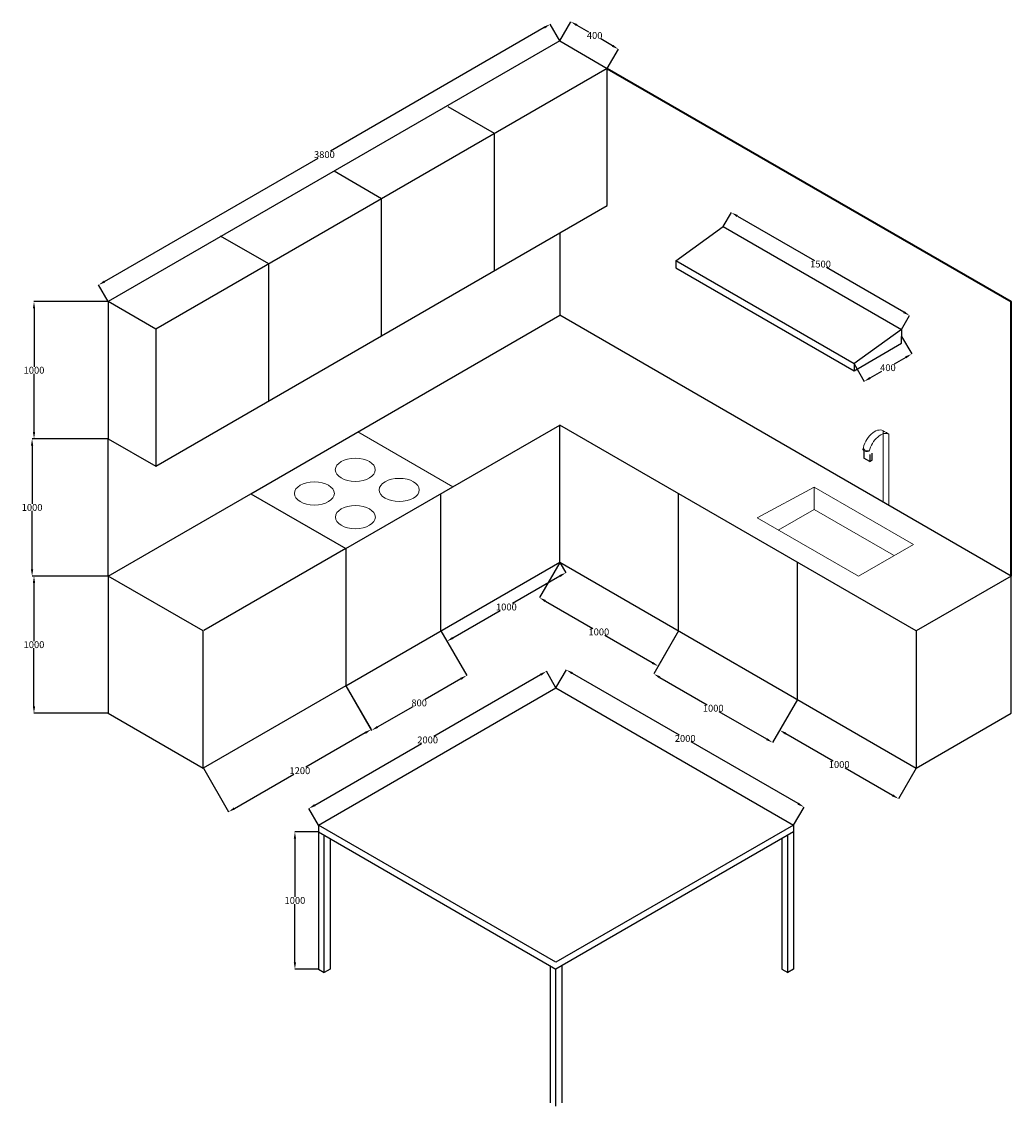
# Model space of a CAD drawing. Units: millimetres. Extents: x -3536 to 3677, y -3825 to 4079.
import ezdxf

# ---------------------------------------------------------------- set-up
doc = ezdxf.new("R2010")
doc.units = ezdxf.units.MM
doc.header["$MEASUREMENT"] = 0
for name, color, linetype, lineweight in [('A-ANNO-DIMS', 2, 'Continuous', 18), ('A-EQPM', 8, 'Continuous', 18), ('A-FLOR-FIXT', 9, 'Continuous', 18), ('A-FURN', 8, 'Continuous', 25), ('A-FURN-CASE', 7, 'Continuous', 25), ('A-WALL', 7, 'Continuous', 35)]:
    doc.layers.add(name, color=color, linetype=linetype, lineweight=lineweight)
doc.styles.get("Standard").update_dxf_attribs({"font": 'arial.ttf'})
doc.dimstyles.get("Standard").update_dxf_attribs({"dimtxt": 50, "dimasz": 50, "dimexe": 0.18, "dimexo": 0.0625, "dimgap": 0.09, "dimtad": 0, "dimtih": 1, "dimtoh": 1, "dimdec": 0, "dimzin": 0, "dimdsep": 46, "dimtxsty": 'Standard', "dimcen": 0.09, "dimadec": 0, "dimazin": 0, "dimtfac": 1, "dimtdec": 0, "dimtofl": 0, "dimtmove": 0, "dimatfit": 3, "dimfxl": 1, "dimtolj": 1, "dimtzin": 0, "dimarcsym": 0})

# ---------------------------------------------------------------- blocks, each defined once
blk = doc.blocks.new('*D1')
at = {"layer": 'A-ANNO-DIMS', "color": 0, "lineweight": -2, "transparency": 16777216}
for p, q in [((272.2, 4035.8), (-1285.6, 3136.4)), ((385.6, 3939.3), (315.4, 4060.9)), ((-2932.1, 2185.8), (-1374.4, 3085.1)), ((-2905.3, 2039.3), (-2975.5, 2160.9))]:
    blk.add_line(p, q, dxfattribs=at)
at = {"layer": 'A-ANNO-DIMS', "color": 0, "transparency": 16777216}
for points in [[(268, 4043), (276.3, 4028.6), (315.5, 4060.8)], [(-2936.3, 2193), (-2928, 2178.6), (-2975.4, 2160.8)]]:
    blk.add_solid(points, dxfattribs=at)
at = {"layer": 'Defpoints', "color": 0, "transparency": 16777216}
for p in [(315.5, 4060.8), (385.6, 3939.3), (-2905.3, 2039.3)]:
    blk.add_point(p, dxfattribs=at)
at = {"layer": 'A-ANNO-DIMS', "color": 0, "transparency": 16777216, "insert": (-1330, 3110.8), "char_height": 50, "attachment_point": 5}
blk.add_mtext('\\A1;3800', dxfattribs=at)
blk = doc.blocks.new('*D2')
at = {"layer": 'A-ANNO-DIMS', "color": 0, "lineweight": -2, "transparency": 16777216}
for p, q in [((-1173.2, -760.8), (-989.3, -1079.3)), ((-1032.7, -1104.1), (-1464.6, -1353.5)), ((-2212.4, -1360.8), (-2028.5, -1679.3)), ((-1985.3, -1654.1), (-1553.4, -1404.8))]:
    blk.add_line(p, q, dxfattribs=at)
at = {"layer": 'A-ANNO-DIMS', "color": 0, "transparency": 16777216}
for points in [[(-1036.9, -1096.9), (-1028.5, -1111.3), (-989.4, -1079.1)], [(-1989.5, -1646.9), (-1981.2, -1661.3), (-2028.6, -1679.1)]]:
    blk.add_solid(points, dxfattribs=at)
at = {"layer": 'Defpoints', "color": 0, "transparency": 16777216}
for p in [(-1173.2, -760.7), (-989.4, -1079.1), (-2212.5, -1360.7)]:
    blk.add_point(p, dxfattribs=at)
at = {"layer": 'A-ANNO-DIMS', "color": 0, "transparency": 16777216, "insert": (-1509, -1379.1), "char_height": 50, "attachment_point": 5}
blk.add_mtext('\\A1;1200', dxfattribs=at)
blk = doc.blocks.new('*D3')
at = {"layer": 'A-ANNO-DIMS', "color": 0, "lineweight": -2, "transparency": 16777216}
for p, q in [((-480.4, -360.8), (-292.9, -685.5)), ((-336.3, -710.3), (-595.1, -859.7)), ((-1173.2, -760.8), (-985.8, -1085.5)), ((-942.5, -1060.3), (-683.8, -910.9))]:
    blk.add_line(p, q, dxfattribs=at)
at = {"layer": 'A-ANNO-DIMS', "color": 0, "transparency": 16777216}
for points in [[(-340.5, -703.1), (-332.2, -717.5), (-293, -685.3)], [(-946.7, -1053.1), (-938.4, -1067.5), (-985.8, -1085.3)]]:
    blk.add_solid(points, dxfattribs=at)
at = {"layer": 'Defpoints', "color": 0, "transparency": 16777216}
for p in [(-480.4, -360.7), (-293, -685.3), (-1173.2, -760.7)]:
    blk.add_point(p, dxfattribs=at)
at = {"layer": 'A-ANNO-DIMS', "color": 0, "transparency": 16777216, "insert": (-639.4, -885.3), "char_height": 50, "attachment_point": 5}
blk.add_mtext('\\A1;800', dxfattribs=at)
blk = doc.blocks.new('*D4')
at = {"layer": 'A-ANNO-DIMS', "color": 0, "lineweight": -2, "transparency": 16777216}
for p, q in [((385.6, 139.2), (429.3, 63.6)), ((385.9, 38.8), (40.6, -160.6)), ((-393.5, -411.2), (-48.2, -211.9)), ((-480.4, -360.8), (-436.7, -436.4))]:
    blk.add_line(p, q, dxfattribs=at)
at = {"layer": 'A-ANNO-DIMS', "color": 0, "transparency": 16777216}
for points in [[(381.7, 46), (390.1, 31.5), (429.2, 63.8)], [(-397.7, -404), (-389.4, -418.5), (-436.8, -436.2)]]:
    blk.add_solid(points, dxfattribs=at)
at = {"layer": 'Defpoints', "color": 0, "transparency": 16777216}
for p in [(385.6, 139.3), (429.2, 63.8), (-480.4, -360.7)]:
    blk.add_point(p, dxfattribs=at)
at = {"layer": 'A-ANNO-DIMS', "color": 0, "transparency": 16777216, "insert": (-3.8, -186.2), "char_height": 50, "attachment_point": 5}
blk.add_mtext('\\A1;1000', dxfattribs=at)
blk = doc.blocks.new('*D5')
at = {"layer": 'A-ANNO-DIMS', "color": 0, "lineweight": -2, "transparency": 16777216}
for p, q in [((385.6, 139.2), (237.1, -118)), ((280.5, -142.8), (625.8, -342.2)), ((1059.9, -592.8), (714.6, -393.5)), ((1251.6, -360.8), (1103.1, -618))]:
    blk.add_line(p, q, dxfattribs=at)
at = {"layer": 'A-ANNO-DIMS', "color": 0, "transparency": 16777216}
for points in [[(284.7, -135.6), (276.3, -150.1), (237.2, -117.8)], [(1064.1, -585.6), (1055.7, -600.1), (1103.2, -617.8)]]:
    blk.add_solid(points, dxfattribs=at)
at = {"layer": 'Defpoints', "color": 0, "transparency": 16777216}
for p in [(385.6, 139.3), (1251.6, -360.7), (1103.2, -617.8)]:
    blk.add_point(p, dxfattribs=at)
at = {"layer": 'A-ANNO-DIMS', "color": 0, "transparency": 16777216, "insert": (670.2, -367.8), "char_height": 50, "attachment_point": 5}
blk.add_mtext('\\A1;1000', dxfattribs=at)
blk = doc.blocks.new('*D6')
at = {"layer": 'A-ANNO-DIMS', "color": 0, "lineweight": -2, "transparency": 16777216}
for p, q in [((1251.6, -360.8), (1070.7, -674.1)), ((1114.1, -699), (1459.4, -898.4)), ((2117.6, -860.8), (1936.7, -1174.1)), ((1893.5, -1149), (1548.2, -949.6))]:
    blk.add_line(p, q, dxfattribs=at)
at = {"layer": 'A-ANNO-DIMS', "color": 0, "transparency": 16777216}
for points in [[(1118.3, -691.8), (1109.9, -706.2), (1070.8, -674)], [(1897.7, -1141.8), (1889.4, -1156.2), (1936.8, -1174)]]:
    blk.add_solid(points, dxfattribs=at)
at = {"layer": 'Defpoints', "color": 0, "transparency": 16777216}
for p in [(1251.6, -360.7), (2117.7, -860.7), (1936.8, -1174)]:
    blk.add_point(p, dxfattribs=at)
at = {"layer": 'A-ANNO-DIMS', "color": 0, "transparency": 16777216, "insert": (1503.8, -924), "char_height": 50, "attachment_point": 5}
blk.add_mtext('\\A1;1000', dxfattribs=at)
blk = doc.blocks.new('*D7')
at = {"layer": 'A-ANNO-DIMS', "color": 0, "lineweight": -2, "transparency": 16777216}
for p, q in [((2117.6, -860.8), (1988.6, -1084.2)), ((2032, -1109.1), (2377.4, -1308.4)), ((2811.5, -1559.1), (2466.1, -1359.7)), ((2983.7, -1360.8), (2854.7, -1584.2))]:
    blk.add_line(p, q, dxfattribs=at)
at = {"layer": 'A-ANNO-DIMS', "color": 0, "transparency": 16777216}
for points in [[(2036.2, -1101.8), (2027.9, -1116.3), (1988.7, -1084.1)], [(2815.6, -1551.8), (2807.3, -1566.3), (2854.8, -1584.1)]]:
    blk.add_solid(points, dxfattribs=at)
at = {"layer": 'Defpoints', "color": 0, "transparency": 16777216}
for p in [(2117.7, -860.7), (2983.7, -1360.7), (2854.8, -1584.1)]:
    blk.add_point(p, dxfattribs=at)
at = {"layer": 'A-ANNO-DIMS', "color": 0, "transparency": 16777216, "insert": (2421.8, -1334.1), "char_height": 50, "attachment_point": 5}
blk.add_mtext('\\A1;1000', dxfattribs=at)
blk = doc.blocks.new('*D8')
at = {"layer": 'A-ANNO-DIMS', "color": 0, "lineweight": -2, "transparency": 16777216}
for p, q in [((-2905.3, 39.3), (-3447, 39.3)), ((-3446.8, -10.7), (-3446.8, -435.1)), ((-3446.8, -910.7), (-3446.8, -486.4)), ((-2905.3, -960.7), (-3447, -960.7))]:
    blk.add_line(p, q, dxfattribs=at)
at = {"layer": 'A-ANNO-DIMS', "color": 0, "transparency": 16777216}
for points in [[(-3455.1, -10.7), (-3438.4, -10.7), (-3446.8, 39.3)], [(-3455.1, -910.7), (-3438.4, -910.7), (-3446.8, -960.7)]]:
    blk.add_solid(points, dxfattribs=at)
at = {"layer": 'Defpoints', "color": 0, "transparency": 16777216}
for p in [(-3446.8, 39.3), (-2905.3, 39.3), (-2905.3, -960.7)]:
    blk.add_point(p, dxfattribs=at)
at = {"layer": 'A-ANNO-DIMS', "color": 0, "transparency": 16777216, "insert": (-3446.8, -460.7), "char_height": 50, "attachment_point": 5}
blk.add_mtext('\\A1;1000', dxfattribs=at)
blk = doc.blocks.new('*D9')
at = {"layer": 'A-ANNO-DIMS', "color": 0, "lineweight": -2, "transparency": 16777216}
for p, q in [((-2905.3, 1039.3), (-3460.8, 1039.3)), ((-3460.6, 989.3), (-3460.6, 564.9)), ((-3460.6, 89.3), (-3460.6, 513.6)), ((-2905.3, 39.3), (-3460.8, 39.3))]:
    blk.add_line(p, q, dxfattribs=at)
at = {"layer": 'A-ANNO-DIMS', "color": 0, "transparency": 16777216}
for points in [[(-3469, 989.3), (-3452.3, 989.3), (-3460.6, 1039.3)], [(-3469, 89.3), (-3452.3, 89.3), (-3460.6, 39.3)]]:
    blk.add_solid(points, dxfattribs=at)
at = {"layer": 'Defpoints', "color": 0, "transparency": 16777216}
for p in [(-3460.6, 1039.3), (-2905.3, 1039.3), (-2905.3, 39.3)]:
    blk.add_point(p, dxfattribs=at)
at = {"layer": 'A-ANNO-DIMS', "color": 0, "transparency": 16777216, "insert": (-3460.6, 539.3), "char_height": 50, "attachment_point": 5}
blk.add_mtext('\\A1;1000', dxfattribs=at)
blk = doc.blocks.new('*D10')
at = {"layer": 'A-ANNO-DIMS', "color": 0, "lineweight": -2, "transparency": 16777216}
for p, q in [((-2905.3, 2039.3), (-3446.8, 2039.3)), ((-3446.6, 1989.3), (-3446.6, 1564.9)), ((-3446.6, 1089.3), (-3446.6, 1513.6)), ((-2905.3, 1039.3), (-3446.8, 1039.3))]:
    blk.add_line(p, q, dxfattribs=at)
at = {"layer": 'A-ANNO-DIMS', "color": 0, "transparency": 16777216}
for points in [[(-3455, 1989.3), (-3438.3, 1989.3), (-3446.6, 2039.3)], [(-3455, 1089.3), (-3438.3, 1089.3), (-3446.6, 1039.3)]]:
    blk.add_solid(points, dxfattribs=at)
at = {"layer": 'Defpoints', "color": 0, "transparency": 16777216}
for p in [(-3446.6, 2039.3), (-2905.3, 2039.3), (-2905.3, 1039.3)]:
    blk.add_point(p, dxfattribs=at)
at = {"layer": 'A-ANNO-DIMS', "color": 0, "transparency": 16777216, "insert": (-3446.6, 1539.3), "char_height": 50, "attachment_point": 5}
blk.add_mtext('\\A1;1000', dxfattribs=at)
blk = doc.blocks.new('*D11')
at = {"layer": 'A-ANNO-DIMS', "color": 0, "lineweight": -2, "transparency": 16777216}
for p, q in [((1577.5, 2585.9), (1636.6, 2688.1)), ((1679.8, 2663), (2241.6, 2338.6)), ((2892.2, 1963), (2330.4, 2287.3)), ((2876.6, 1835.9), (2935.6, 1938.1))]:
    blk.add_line(p, q, dxfattribs=at)
at = {"layer": 'A-ANNO-DIMS', "color": 0, "transparency": 16777216}
for points in [[(1684, 2670.2), (1675.6, 2655.7), (1636.5, 2688)], [(2896.4, 1970.2), (2888.1, 1955.7), (2935.5, 1938)]]:
    blk.add_solid(points, dxfattribs=at)
at = {"layer": 'Defpoints', "color": 0, "transparency": 16777216}
for p in [(1577.5, 2585.8), (2935.5, 1938), (2876.5, 1835.8)]:
    blk.add_point(p, dxfattribs=at)
at = {"layer": 'A-ANNO-DIMS', "color": 0, "transparency": 16777216, "insert": (2286, 2313), "char_height": 50, "attachment_point": 5}
blk.add_mtext('\\A1;1500', dxfattribs=at)
blk = doc.blocks.new('*D12')
at = {"layer": 'A-ANNO-DIMS', "color": 0, "lineweight": -2, "transparency": 16777216}
for p, q in [((2876.6, 1785.7), (2950.5, 1657.7)), ((2530.2, 1585.7), (2604.1, 1457.7)), ((2907.1, 1632.9), (2821.6, 1583.5)), ((2647.3, 1482.9), (2732.8, 1532.2))]:
    blk.add_line(p, q, dxfattribs=at)
at = {"layer": 'A-ANNO-DIMS', "color": 0, "transparency": 16777216}
for points in [[(2902.9, 1640.1), (2911.3, 1625.7), (2950.4, 1657.9)], [(2643.1, 1490.1), (2651.5, 1475.7), (2604, 1457.9)]]:
    blk.add_solid(points, dxfattribs=at)
at = {"layer": 'Defpoints', "color": 0, "transparency": 16777216}
for p in [(2876.5, 1785.8), (2530.1, 1585.8), (2604, 1457.9)]:
    blk.add_point(p, dxfattribs=at)
at = {"layer": 'A-ANNO-DIMS', "color": 0, "transparency": 16777216, "insert": (2777.2, 1557.9), "char_height": 50, "attachment_point": 5}
blk.add_mtext('\\A1;400', dxfattribs=at)
blk = doc.blocks.new('*D13')
at = {"layer": 'A-ANNO-DIMS', "color": 0, "lineweight": -2, "transparency": 16777216}
for p, q in [((385.6, 3939.3), (466.5, 4079.3)), ((509.7, 4054.1), (595.2, 4004.7)), ((769.5, 3904.1), (683.9, 3953.5)), ((732.1, 3739.3), (812.9, 3879.3))]:
    blk.add_line(p, q, dxfattribs=at)
at = {"layer": 'A-ANNO-DIMS', "color": 0, "transparency": 16777216}
for points in [[(513.8, 4061.3), (505.5, 4046.9), (466.4, 4079.1)], [(773.6, 3911.3), (765.3, 3896.9), (812.8, 3879.1)]]:
    blk.add_solid(points, dxfattribs=at)
at = {"layer": 'Defpoints', "color": 0, "transparency": 16777216}
for p in [(385.6, 3939.3), (812.8, 3879.1), (732, 3739.3)]:
    blk.add_point(p, dxfattribs=at)
at = {"layer": 'A-ANNO-DIMS', "color": 0, "transparency": 16777216, "insert": (639.6, 3979.1), "char_height": 50, "attachment_point": 5}
blk.add_mtext('\\A1;400', dxfattribs=at)
blk = doc.blocks.new('*D14')
at = {"layer": 'A-ANNO-DIMS', "color": 0, "lineweight": -2, "transparency": 16777216}
for p, q in [((245.3, -680.1), (-533.1, -1129.5)), ((357.9, -775.1), (288.5, -654.9)), ((-1400.2, -1630.1), (-621.8, -1180.7)), ((-1374.2, -1775.1), (-1443.6, -1654.9))]:
    blk.add_line(p, q, dxfattribs=at)
at = {"layer": 'A-ANNO-DIMS', "color": 0, "transparency": 16777216}
for points in [[(241.1, -672.9), (249.4, -687.3), (288.6, -655.1)], [(-1404.3, -1622.9), (-1396, -1637.3), (-1443.5, -1655.1)]]:
    blk.add_solid(points, dxfattribs=at)
at = {"layer": 'Defpoints', "color": 0, "transparency": 16777216}
for p in [(288.6, -655.1), (357.9, -775.1), (-1374.2, -1775.1)]:
    blk.add_point(p, dxfattribs=at)
at = {"layer": 'A-ANNO-DIMS', "color": 0, "transparency": 16777216, "insert": (-577.5, -1155.1), "char_height": 50, "attachment_point": 5}
blk.add_mtext('\\A1;2000', dxfattribs=at)
blk = doc.blocks.new('*D15')
at = {"layer": 'A-ANNO-DIMS', "color": 0, "lineweight": -2, "transparency": 16777216}
for p, q in [((357.9, -775.1), (433.5, -644.1)), ((476.7, -669.3), (1255.1, -1118.7)), ((2122.2, -1619.3), (1343.8, -1169.9)), ((2090, -1775.1), (2165.6, -1644.1))]:
    blk.add_line(p, q, dxfattribs=at)
at = {"layer": 'A-ANNO-DIMS', "color": 0, "transparency": 16777216}
for points in [[(480.9, -662.1), (472.6, -676.5), (433.4, -644.3)], [(2126.4, -1612.1), (2118, -1626.5), (2165.5, -1644.3)]]:
    blk.add_solid(points, dxfattribs=at)
at = {"layer": 'Defpoints', "color": 0, "transparency": 16777216}
for p in [(357.9, -775.1), (2165.5, -1644.3), (2089.9, -1775.1)]:
    blk.add_point(p, dxfattribs=at)
at = {"layer": 'A-ANNO-DIMS', "color": 0, "transparency": 16777216, "insert": (1299.5, -1144.3), "char_height": 50, "attachment_point": 5}
blk.add_mtext('\\A1;2000', dxfattribs=at)
blk = doc.blocks.new('*D16')
at = {"layer": 'A-ANNO-DIMS', "color": 0, "lineweight": -2, "transparency": 16777216}
for p, q in [((-1374.2, -1825.1), (-1545.1, -1825.1)), ((-1544.9, -1875.1), (-1544.9, -2299.5)), ((-1544.9, -2775.1), (-1544.9, -2350.8)), ((-1374.2, -2825.1), (-1545.1, -2825.1))]:
    blk.add_line(p, q, dxfattribs=at)
at = {"layer": 'A-ANNO-DIMS', "color": 0, "transparency": 16777216}
for points in [[(-1553.3, -1875.1), (-1536.6, -1875.1), (-1544.9, -1825.1)], [(-1553.3, -2775.1), (-1536.6, -2775.1), (-1544.9, -2825.1)]]:
    blk.add_solid(points, dxfattribs=at)
at = {"layer": 'Defpoints', "color": 0, "transparency": 16777216}
for p in [(-1374.2, -1825.1), (-1544.9, -2825.1), (-1374.2, -2825.1)]:
    blk.add_point(p, dxfattribs=at)
at = {"layer": 'A-ANNO-DIMS', "color": 0, "transparency": 16777216, "insert": (-1544.9, -2325.1), "char_height": 50, "attachment_point": 5}
blk.add_mtext('\\A1;1000', dxfattribs=at)

msp = doc.modelspace()

# ---------------------------------------------------------------- linework, layer by layer
at = {"layer": 'A-EQPM'}
msp.add_line((-393.8, 689.3), (-1086.6, 1089.3), dxfattribs=at)
for centre in [(-1104.8, 813.4), (-1403.2, 641.1), (-784.6, 667.1), (-1104.3, 468.6)]:
    msp.add_ellipse(centre, major_axis=(-145.9, 0), ratio=0.57735, dxfattribs=at)
at = {"layer": 'A-FLOR-FIXT'}
for p, q in [((2741.6, 1098.3), (2741.6, 579)), ((2741.6, 1098.3), (2749.5, 1093.8)), ((2784.9, 1073.3), (2771.1, 1081.3)), ((2784.9, 1073.3), (2784.9, 554)), ((1824.6, 462.5), (2240.3, 687.6)), ((2240.3, 687.6), (2963.9, 269.8)), ((2240.3, 687.6), (2240.3, 525.3)), ((2240.3, 525.3), (1978.2, 374)), ((2240.3, 525.3), (2816.8, 192.5)), ((2562.1, 37.9), (1824.6, 462.5)), ((2963.9, 269.8), (2562.1, 37.9))]:
    msp.add_line(p, q, dxfattribs=at)
for centre, start, end in [((2624.3, 980.2), 212.85651, 299.04765), ((2627.8, 986.2), 207.18602, 294.88734)]:
    msp.add_arc(centre, 34.6, start, end, dxfattribs=at)
for centre, end_param in [((2680.4, 992.2), 5.313627), ((2723.7, 967.2), 5.189776)]:
    msp.add_ellipse(centre, major_axis=(-61.2, -106.1), ratio=0.57735, start_param=3.141593, end_param=end_param, dxfattribs=at)
msp.add_open_spline([(2771.1, 1081.3), (2763.9, 1085.4), (2756.7, 1089.6), (2749.5, 1093.8)], degree=3, dxfattribs=at)
at = {"layer": 'A-FURN'}
for p, q in [((1231.1, 2335.8), (1577.5, 2585.8)), ((1577.5, 2585.8), (2876.5, 1835.8)), ((2530.1, 1585.8), (1231.1, 2335.8)), ((1231.1, 2335.8), (1231.1, 2285.8)), ((1231.1, 2285.8), (2530.1, 1535.8)), ((2876.5, 1835.8), (2876.5, 1785.8)), ((2876.5, 1735.8), (2876.5, 1785.8)), ((2530.1, 1535.8), (2876.5, 1735.8)), ((2530.1, 1585.8), (2530.1, 1535.8)), ((-1374.2, -1775.1), (357.9, -775.1)), ((357.9, -775.1), (2089.9, -1775.1)), ((357.9, -2775.1), (-1374.2, -1775.1)), ((-1374.2, -1775.1), (-1374.2, -1825.1)), ((2089.9, -1775.1), (357.9, -2775.1)), ((2089.9, -1775.1), (2089.9, -1825.1)), ((-1374.2, -1825.1), (357.9, -2825.1)), ((-1374.2, -1825.1), (-1374.2, -2825.1)), ((-1330.9, -2850.1), (-1330.9, -1850.1)), ((-1287.6, -1875.1), (-1287.6, -2825.1)), ((2089.9, -1825.1), (357.9, -2825.1)), ((2003.3, -1875.1), (2003.3, -2825.1)), ((2046.6, -2850.1), (2046.6, -1850.1)), ((2089.9, -1825.1), (2089.9, -2825.1)), ((-1374.2, -2825.1), (-1330.9, -2850.1)), ((-1287.6, -2825.1), (-1330.9, -2850.1)), ((314.6, -2800.1), (314.6, -3800.1)), ((357.9, -3825.1), (357.9, -2825.1)), ((401.2, -2800.1), (401.2, -3800.1)), ((2003.3, -2825.1), (2046.6, -2850.1)), ((2089.9, -2825.1), (2046.6, -2850.1))]:
    msp.add_line(p, q, dxfattribs=at)
at = {"layer": 'A-FURN-CASE'}
for p, q in [((385.6, 3939.3), (-2905.3, 2039.3)), ((385.6, 3939.3), (732, 3739.3)), ((732, 3739.3), (-2558.9, 1839.3)), ((732, 2739.3), (732, 3739.3)), ((-90.7, 3264.3), (-427, 3458.4)), ((-90.7, 2264.3), (-90.7, 3264.3)), ((-913.4, 2789.3), (-1259.8, 2989.3)), ((-913.4, 1789.3), (-913.4, 2789.3)), ((-2558.9, 839.3), (732, 2739.3)), ((385.6, 2539.3), (385.6, 1939.3)), ((-1736.1, 2314.3), (-2086.3, 2516.4)), ((-1736.1, 1314.3), (-1736.1, 2314.3)), ((-2905.3, 2039.3), (-2905.3, 1039.3)), ((-2558.9, 1839.3), (-2905.3, 2039.3)), ((-1866, 639.3), (385.6, 1939.3)), ((3676.5, 39.3), (385.6, 1939.3)), ((-2558.9, 1839.3), (-2558.9, 839.3)), ((2876.3, 1836.3), (2529.9, 1586.3)), ((-1173.2, 239.3), (385.6, 1139.3)), ((385.6, 139.3), (385.6, 1139.3)), ((2983.7, -360.7), (385.6, 1139.3)), ((-2905.3, 39.3), (-2905.3, 1039.3)), ((-2905.3, 1039.3), (-2558.9, 839.3)), ((2602.6, 949.3), (2602.6, 899.3)), ((2645.9, 874.3), (2602.6, 899.3)), ((2645.9, 924.3), (2645.9, 874.3)), ((2645.9, 874.3), (2663.3, 884.3)), ((2663.3, 884.3), (2663.3, 934.3)), ((-2905.3, 39.3), (-1866, 639.3)), ((-1866, 639.3), (-1173.2, 239.3)), ((-480.4, -360.7), (-480.4, 639.3)), ((1251.6, -360.7), (1251.6, 639.3)), ((-1173.2, 239.3), (-2207.9, -358.1)), ((-1173.2, 239.3), (-1173.2, -760.7)), ((-1173.2, -760.7), (385.6, 139.3)), ((385.6, 139.3), (2983.7, -1360.7)), ((2117.7, -860.7), (2117.7, 139.3)), ((-2212.5, -360.7), (-2905.3, 39.3)), ((-2905.3, 39.3), (-2905.3, -960.7)), ((3676.5, 39.3), (2983.7, -360.7)), ((3676.5, -960.7), (3676.5, 39.3)), ((-2212.5, -1360.7), (-2212.5, -360.7)), ((2983.7, -360.7), (2983.7, -1360.7)), ((-1173.2, -760.7), (-2212.5, -1360.7)), ((-2905.3, -960.7), (-2212.5, -1360.7)), ((2983.7, -1360.7), (3676.5, -960.7))]:
    msp.add_line(p, q, dxfattribs=at)
at = {"layer": 'A-WALL'}
for p in [(732, 3739.3), (3676.5, 39.3)]:
    msp.add_line(p, (3676.5, 2039.3), dxfattribs=at)

# ---------------------------------------------------------------- dimensions: what is measured, and where the dimension line sits
at = {"layer": 'A-ANNO-DIMS'}
for p1, p2, distance, override, picture, middle in [((-2905.3, 2039.3), (385.6, 3939.3), 140.3, {"dimtxt": 50, "dimasz": 50, "dimclrd": 0, "dimclre": 0, "dimclrt": 0}, '*D1', (-1330, 3110.8)), ((385.6, 3939.3), (732, 3739.3), 161.5, {"dimclrd": 0, "dimclre": 0, "dimclrt": 0}, '*D13', (639.6, 3979.1)), ((1577.5, 2585.8), (2876.5, 1835.8), 118, {"dimclrd": 0, "dimclre": 0, "dimclrt": 0}, '*D11', (2286, 2313)), ((-2905.3, 1039.3), (-2905.3, 2039.3), 541.4, {"dimclrd": 0, "dimclre": 0, "dimclrt": 0}, '*D10', (-3446.6, 1539.3)), ((2876.5, 1785.8), (2530.1, 1585.8), 147.7, {"dimclrd": 0, "dimclre": 0, "dimclrt": 0}, '*D12', (2777.2, 1557.9)), ((-2905.3, 39.3), (-2905.3, 1039.3), 555.4, {"dimclrd": 0, "dimclre": 0, "dimclrt": 0}, '*D9', (-3460.6, 539.3)), ((-480.4, -360.7), (385.6, 139.3), -87.2, {"dimclrd": 0, "dimclre": 0, "dimclrt": 0}, '*D4', (-3.8, -186.2)), ((385.6, 139.3), (1251.6, -360.7), -296.9, {"dimclrd": 0, "dimclre": 0, "dimclrt": 0}, '*D5', (670.2, -367.8)), ((-2905.3, -960.7), (-2905.3, 39.3), 541.5, {"dimclrd": 0, "dimclre": 0, "dimclrt": 0}, '*D8', (-3446.8, -460.7)), ((-1173.2, -760.7), (-480.4, -360.7), -374.8, {"dimclrd": 0, "dimclre": 0, "dimclrt": 0}, '*D3', (-639.4, -885.3)), ((1251.6, -360.7), (2117.7, -860.7), -361.7, {"dimclrd": 0, "dimclre": 0, "dimclrt": 0}, '*D6', (1503.8, -924)), ((-1374.2, -1775.1), (357.9, -775.1), 138.6, {"dimclrd": 0, "dimclre": 0, "dimclrt": 0}, '*D14', (-577.5, -1155.1)), ((357.9, -775.1), (2089.9, -1775.1), 151.1, {"dimclrd": 0, "dimclre": 0, "dimclrt": 0}, '*D15', (1299.5, -1144.3)), ((-2212.5, -1360.7), (-1173.2, -760.7), -367.6, {"dimclrd": 0, "dimclre": 0, "dimclrt": 0}, '*D2', (-1509, -1379.1)), ((2117.7, -860.7), (2983.7, -1360.7), -257.9, {"dimclrd": 0, "dimclre": 0, "dimclrt": 0}, '*D7', (2421.8, -1334.1)), ((-1374.2, -1825.1), (-1374.2, -2825.1), -170.8, {"dimclrd": 0, "dimclre": 0, "dimclrt": 0}, '*D16', (-1544.9, -2325.1))]:
    dim = msp.add_aligned_dim(p1=p1, p2=p2, distance=distance, dimstyle='Standard', override=override, dxfattribs=at)
    dim.commit()
    dim.dimension.update_dxf_attribs({"geometry": picture, "text_midpoint": middle})

doc.saveas('drawing.dxf')
